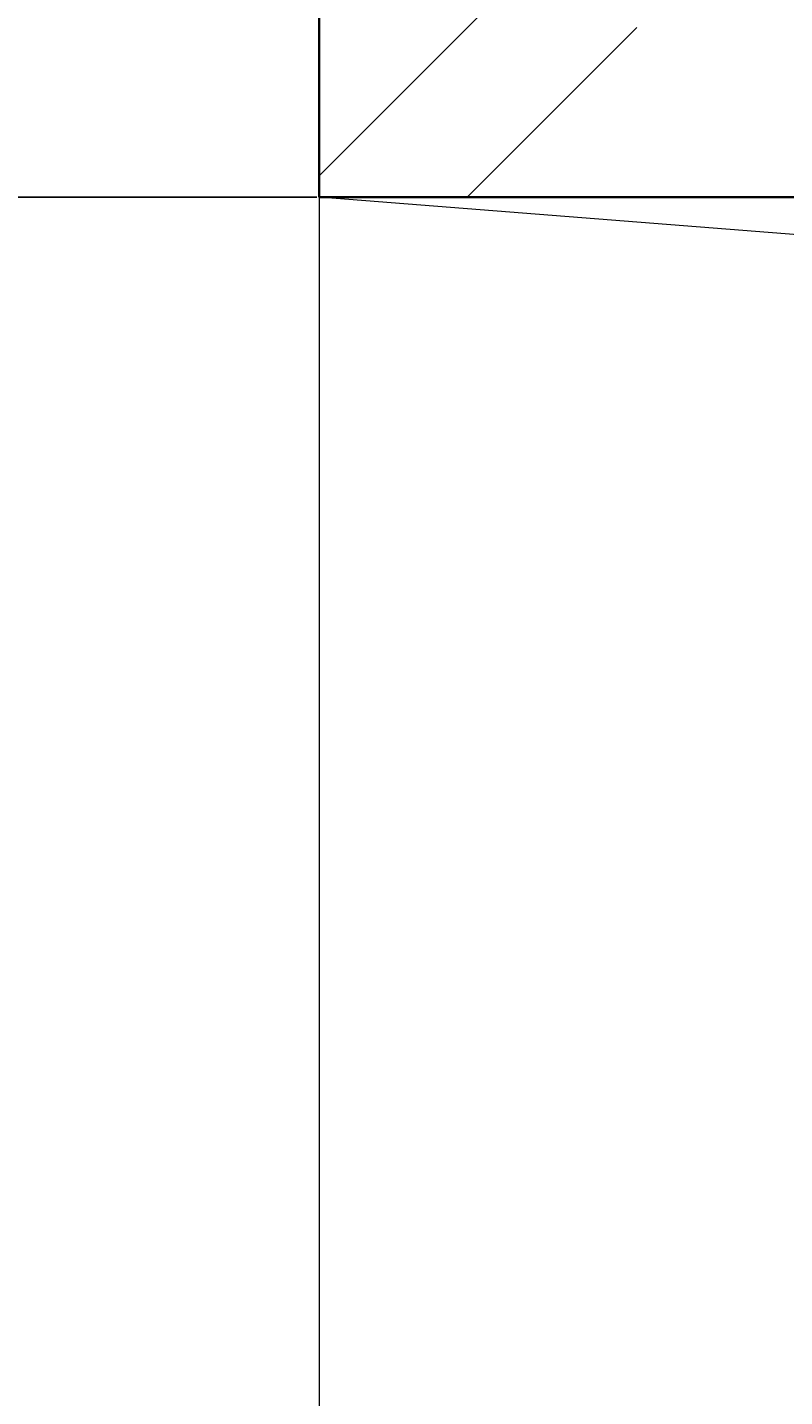
# Model space of a CAD drawing. Units: inches. Extents: x 1885 to 2748, y 783 to 2421.
# Tile 57 of 117: x 2009 to 2029, y 1850 to 1886. Entities that reach past the tile are written whole.
import ezdxf

# ---------------------------------------------------------------- set-up
doc = ezdxf.new("R2010")
doc.units = ezdxf.units.IN
for name, color, linetype, lineweight in [('A-ANNO-DIMS', 2, 'Continuous', 18), ('A-FLOR-OPEN', 8, 'Continuous', 13), ('A-WALL', 7, 'Continuous', 35)]:
    doc.layers.add(name, color=color, linetype=linetype, lineweight=lineweight)
doc.layers.add('A-WALL-PATT', color=85, linetype='Continuous', lineweight=13, true_color=0x58ba48)
doc.styles.get("Standard").update_dxf_attribs({"font": 'arial.ttf'})
doc.dimstyles.get("Standard").update_dxf_attribs({"dimtxt": 0.18, "dimasz": 0.18, "dimexe": 0.18, "dimexo": 0.0625, "dimgap": 0.09, "dimtad": 0, "dimtih": 1, "dimtoh": 1, "dimdec": 4, "dimzin": 0, "dimdsep": 46, "dimtxsty": 'Standard', "dimcen": 0.09, "dimadec": 0, "dimazin": 0, "dimtfac": 1, "dimtdec": 4, "dimtofl": 0, "dimtmove": 0, "dimatfit": 3, "dimfxl": 1, "dimtolj": 1, "dimtzin": 0, "dimarcsym": 0})

# ---------------------------------------------------------------- blocks, each defined once
blk = doc.blocks.new('*D48')
at = {"layer": 'A-ANNO-DIMS', "color": 0, "lineweight": -2, "transparency": 16777216}
for p, q in [((1980.711, 2348.006), (1902.844, 2348.006)), ((1903.024, 2347.826), (1903.024, 2114.937)), ((1903.024, 1881.686), (1903.024, 2114.574)), ((2016.711, 1881.506), (1902.844, 1881.506))]:
    blk.add_line(p, q, dxfattribs=at)
at = {"layer": 'A-ANNO-DIMS', "color": 0, "transparency": 16777216}
for points in [[(1902.994, 2347.826), (1903.054, 2347.826), (1903.024, 2348.006)], [(1902.994, 1881.686), (1903.054, 1881.686), (1903.024, 1881.506)]]:
    blk.add_solid(points, dxfattribs=at)
at = {"layer": 'Defpoints', "color": 0, "transparency": 16777216}
for p in [(1903.024, 2348.006), (1980.774, 2348.006), (2016.774, 1881.506)]:
    blk.add_point(p, dxfattribs=at)
at = {"layer": 'A-ANNO-DIMS', "color": 0, "transparency": 16777216, "insert": (1903.024, 2114.756), "char_height": 0.18, "attachment_point": 5}
blk.add_mtext('\\A1;466.5', dxfattribs=at)

msp = doc.modelspace()

# ---------------------------------------------------------------- hatches: boundary and pattern name
at = {"layer": 'A-WALL-PATT'}
h = msp.add_hatch(dxfattribs=at)
h.set_pattern_fill('ANSI32', color=256)
h.paths.add_polyline_path([(2007.772, 2318.006), (1980.774, 2318.006), (1980.774, 2281.215), (1985.274, 2281.215), (1985.274, 2313.506), (2007.772, 2313.506), (2007.772, 2315.756)])
h.paths.add_polyline_path([(2094.324, 2318.006), (2067.772, 2318.006), (2067.772, 2313.506), (2094.324, 2313.506), (2094.324, 2315.756)])
h.paths.add_polyline_path([(2131.367, 2315.756), (2131.367, 2318.006), (2131.189, 2318.006), (2112.609, 2318.006), (2112.609, 2313.506), (2117.274, 2313.506), (2117.274, 2255.201), (2121.774, 2255.201), (2121.774, 2313.506), (2131.367, 2313.506)])
h.paths.add_polyline_path([(2190.512, 2318.006), (2155.367, 2318.006), (2155.367, 2313.506), (2169.774, 2313.506), (2169.774, 2229.506), (2121.774, 2229.506), (2121.774, 2233.451), (2119.524, 2233.451), (2117.274, 2233.451), (2117.274, 2201.101), (2121.774, 2201.101), (2121.774, 2225.006), (2169.774, 2225.006), (2169.774, 2165.006), (2306.274, 2165.006), (2306.274, 2066.006), (2310.774, 2066.006), (2344.274, 2066.006), (2486.274, 2066.006), (2486.274, 1886.006), (2483.02, 1886.006), (2483.02, 1881.506), (2486.274, 1881.506), (2486.274, 1880.678), (2490.774, 1880.678), (2490.774, 2070.506), (2344.274, 2070.506), (2310.774, 2070.506), (2310.774, 2165.006), (2310.774, 2173.636), (2308.524, 2173.636), (2306.274, 2173.636), (2306.274, 2169.506), (2174.274, 2169.506), (2174.274, 2313.506), (2190.512, 2313.506), (2190.512, 2315.756)])
h.paths.add_polyline_path([(1985.274, 2221.215), (1980.774, 2221.215), (1980.774, 2165.006), (1992.774, 2165.006), (1992.774, 2141.927), (1997.274, 2141.927), (1997.274, 2165.006), (2117.274, 2165.006), (2117.274, 2163.126), (2121.774, 2163.126), (2121.774, 2172.734), (2119.524, 2172.734), (2117.274, 2172.734), (2117.274, 2169.506), (1985.274, 2169.506)])
h.paths.add_polyline_path([(1997.274, 2105.927), (1992.774, 2105.927), (1992.774, 2070.506), (2016.774, 2070.506), (2016.774, 2059.123), (2019.024, 2059.123), (2021.274, 2059.123), (2021.274, 2070.506), (2117.274, 2070.506), (2117.274, 2022.506), (2114.423, 2022.506), (2114.423, 2018.006), (2123.627, 2018.006), (2123.627, 2020.256), (2123.627, 2022.506), (2121.774, 2022.506), (2121.774, 2142.587), (2119.524, 2142.587), (2117.274, 2142.587), (2117.274, 2075.006), (1997.274, 2075.006)])
h.paths.add_polyline_path([(2092.029, 2020.256), (2092.029, 2022.506), (2021.274, 2022.506), (2021.274, 2035.123), (2016.774, 2035.123), (2016.774, 2018.006), (2016.774, 1978.784), (2021.274, 1978.784), (2021.274, 2018.006), (2092.029, 2018.006)])
h.paths.add_polyline_path([(2260.938, 2022.506), (2153.105, 2022.506), (2153.105, 2020.256), (2153.105, 2018.006), (2155.274, 2018.006), (2155.274, 1886.006), (2107.629, 1886.006), (2107.629, 1881.506), (2182.911, 1881.506), (2182.911, 1883.756), (2182.911, 1886.006), (2159.774, 1886.006), (2159.774, 2018.006), (2260.938, 2018.006), (2260.938, 2020.256)])
h.paths.add_polyline_path([(2047.629, 1883.756), (2047.629, 1886.006), (2021.274, 1886.006), (2021.274, 1918.784), (2019.024, 1918.784), (2016.774, 1918.784), (2016.774, 1881.506), (2047.629, 1881.506)])
h.paths.add_polyline_path([(2306.361, 1883.756), (2306.361, 1886.006), (2296.274, 1886.006), (2296.274, 1982.006), (2316.535, 1982.006), (2316.535, 1984.256), (2316.535, 1986.506), (2296.274, 1986.506), (2296.274, 2022.506), (2289.276, 2022.506), (2289.276, 2018.006), (2291.774, 2018.006), (2291.774, 1886.006), (2242.911, 1886.006), (2242.911, 1881.506), (2306.361, 1881.506)], flags=17)
h.paths.add_polyline_path([(1985.274, 1843.006), (2021.6, 1843.006), (2021.534, 1845.441), (2021.477, 1847.506), (1980.774, 1847.506), (1980.774, 1809.446), (1985.274, 1809.446)])
h.paths.add_polyline_path([(2131.482, 1845.256), (2131.482, 1847.506), (2081.534, 1847.506), (2081.534, 1843.006), (2117.274, 1843.006), (2117.274, 1784.147), (2119.524, 1784.147), (2121.774, 1784.147), (2121.774, 1843.006), (2131.482, 1843.006)])
h.paths.add_polyline_path([(2203.886, 1847.506), (2155.482, 1847.506), (2155.482, 1843.006), (2169.774, 1843.006), (2169.774, 1759.006), (2121.774, 1759.006), (2121.774, 1761.457), (2117.274, 1761.457), (2117.274, 1730.429), (2121.774, 1730.429), (2121.774, 1754.506), (2177.421, 1754.506), (2177.421, 1756.756), (2177.421, 1759.006), (2174.274, 1759.006), (2174.274, 1843.006), (2203.886, 1843.006)])
h.paths.add_polyline_path([(2335.554, 1845.256), (2335.554, 1847.506), (2239.886, 1847.506), (2239.886, 1843.006), (2306.274, 1843.006), (2306.274, 1759.006), (2199.486, 1759.006), (2199.486, 1754.506), (2310.774, 1754.506), (2310.774, 1843.006), (2335.554, 1843.006)])
h.paths.add_polyline_path([(2348.774, 2022.506), (2344.274, 2022.506), (2344.274, 1986.506), (2341.681, 1986.506), (2341.681, 1982.006), (2344.274, 1982.006), (2344.274, 1886.006), (2330.361, 1886.006), (2330.361, 1881.506), (2361.627, 1881.506), (2361.627, 1883.756), (2361.627, 1886.006), (2348.774, 1886.006)], flags=17)
h.paths.add_polyline_path([(2283.251, 2315.756), (2283.251, 2318.006), (2238.512, 2318.006), (2238.512, 2313.506), (2283.251, 2313.506)], flags=17)
h.paths.add_polyline_path([(2363.274, 2348.006), (2388.677, 2348.006), (2388.677, 2350.256), (2388.677, 2352.506), (2358.774, 2352.506), (2358.774, 2348.006), (2358.774, 2318.006), (2344.481, 2318.006), (2344.481, 2313.506), (2358.774, 2313.506), (2358.774, 2229.506), (2310.774, 2229.506), (2310.774, 2231.952), (2306.274, 2231.952), (2306.274, 2205.611), (2310.774, 2205.611), (2310.774, 2225.006), (2358.774, 2225.006), (2358.774, 2211.506), (2452.329, 2211.506), (2452.329, 2213.756), (2452.329, 2216.006), (2363.274, 2216.006), (2363.274, 2318.006)])
h.paths.add_polyline_path([(2310.774, 2313.506), (2320.481, 2313.506), (2320.481, 2315.756), (2320.481, 2318.006), (2302.728, 2318.006), (2302.728, 2313.506), (2306.274, 2313.506), (2306.274, 2251.076), (2310.774, 2251.076)], flags=17)
h.paths.add_polyline_path([(2490.774, 2352.506), (2486.274, 2352.506), (2448.677, 2352.506), (2448.677, 2348.006), (2486.274, 2348.006), (2486.274, 2318.006), (2486.274, 2216.006), (2481.78, 2216.006), (2481.78, 2211.506), (2486.274, 2211.506), (2486.274, 2165.006), (2493.289, 2165.006), (2493.289, 2167.256), (2493.289, 2169.506), (2490.774, 2169.506), (2490.774, 2313.506), (2494.429, 2313.506), (2494.429, 2318.006), (2490.774, 2318.006)])
h.paths.add_polyline_path([(2534.653, 2318.006), (2515.691, 2318.006), (2515.691, 2313.506), (2534.653, 2313.506), (2534.653, 2315.756)])
h.paths.add_polyline_path([(2618.274, 2318.006), (2594.653, 2318.006), (2594.653, 2313.506), (2613.774, 2313.506), (2613.774, 2281.706), (2618.274, 2281.706)])
h.paths.add_polyline_path([(2618.274, 2221.706), (2613.774, 2221.706), (2613.774, 2169.506), (2554.019, 2169.506), (2554.019, 2165.006), (2613.774, 2165.006), (2613.774, 2152.878), (2618.274, 2152.878)])
h.paths.add_polyline_path([(2618.274, 2128.878), (2616.024, 2128.878), (2613.774, 2128.878), (2613.774, 2117.006), (2529.774, 2117.006), (2529.774, 2165.006), (2532.848, 2165.006), (2532.848, 2169.506), (2522.867, 2169.506), (2522.867, 2165.006), (2525.274, 2165.006), (2525.274, 2117.006), (2525.274, 2112.506), (2525.274, 2108.576), (2529.774, 2108.576), (2529.774, 2112.506), (2613.774, 2112.506), (2613.774, 2080.19), (2618.274, 2080.19)])
h.paths.add_polyline_path([(2618.274, 2044.19), (2616.024, 2044.19), (2613.774, 2044.19), (2613.774, 2015.506), (2529.774, 2015.506), (2529.774, 2088.582), (2527.524, 2088.582), (2525.274, 2088.582), (2525.274, 2011.006), (2613.774, 2011.006), (2613.774, 1956.755), (2618.274, 1956.755)])
h.paths.add_polyline_path([(2618.274, 1881.506), (2618.274, 1896.755), (2613.774, 1896.755), (2613.774, 1881.506), (2613.774, 1847.506), (2592.715, 1847.506), (2592.715, 1843.006), (2613.774, 1843.006), (2613.774, 1765.006), (2613.774, 1760.506), (2609.621, 1760.506), (2609.621, 1756.006), (2613.774, 1756.006), (2613.774, 1660.006), (2608.544, 1660.006), (2608.544, 1655.506), (2613.774, 1655.506), (2613.774, 1508.158), (2618.274, 1508.158)])
h.paths.add_polyline_path([(2565.774, 1843.006), (2568.997, 1843.006), (2568.997, 1847.506), (2490.774, 1847.506), (2490.774, 1849.7), (2488.524, 1849.7), (2486.274, 1849.7), (2486.274, 1847.506), (2477.274, 1847.506), (2477.274, 1838.506), (2477.274, 1821.493), (2486.274, 1821.493), (2486.274, 1838.506), (2561.274, 1838.506), (2561.274, 1765.006), (2486.274, 1765.006), (2486.274, 1786.157), (2477.274, 1786.157), (2477.274, 1765.006), (2477.274, 1756.006), (2486.274, 1756.006), (2565.774, 1756.006), (2585.621, 1756.006), (2585.621, 1758.256), (2585.621, 1760.506), (2565.774, 1760.506), (2565.774, 1765.006)])
h.paths.add_polyline_path([(2486.274, 1651.006), (2561.274, 1651.006), (2561.274, 1567.006), (2486.274, 1567.006), (2486.274, 1591.321), (2477.274, 1591.321), (2477.274, 1567.006), (2477.274, 1558.006), (2477.274, 1555.439), (2481.774, 1555.439), (2481.774, 1558.006), (2568.653, 1558.006), (2568.653, 1560.256), (2568.653, 1562.506), (2565.774, 1562.506), (2565.774, 1655.506), (2584.544, 1655.506), (2584.544, 1657.756), (2584.544, 1660.006), (2565.774, 1660.006), (2486.274, 1660.006), (2477.274, 1660.006), (2477.274, 1651.006), (2477.274, 1632.989), (2486.274, 1632.989)])
h.paths.add_polyline_path([(2449.967, 1883.756), (2449.967, 1886.006), (2421.627, 1886.006), (2421.627, 1881.506), (2449.967, 1881.506)], flags=17)
h.paths.add_polyline_path([(2447.274, 1847.506), (2395.554, 1847.506), (2395.554, 1843.006), (2442.774, 1843.006), (2442.774, 1809.27), (2447.274, 1809.27)])
h.paths.add_polyline_path([(1985.274, 1749.446), (1980.774, 1749.446), (1980.774, 1694.504), (1985.274, 1694.504), (1985.274, 1694.506), (1986.897, 1694.506), (1986.897, 1697.78), (1986.897, 1699.006), (1985.274, 1699.006)])
h.paths.add_polyline_path([(2152.774, 1699.006), (2121.774, 1699.006), (2121.774, 1703.668), (2119.524, 1703.668), (2117.274, 1703.668), (2117.274, 1699.006), (2009.219, 1699.006), (2009.219, 1694.506), (2148.274, 1694.506), (2148.274, 1692.631), (2152.774, 1692.631)])
h.paths.add_polyline_path([(2016.274, 1694.506), (2011.774, 1694.506), (2011.774, 1558.006), (2040.806, 1558.006), (2040.806, 1560.256), (2040.806, 1562.506), (2016.274, 1562.506)])
h.paths.add_polyline_path([(2152.774, 1663.017), (2150.524, 1663.017), (2148.274, 1663.017), (2148.274, 1562.506), (2100.806, 1562.506), (2100.806, 1558.006), (2165.119, 1558.006), (2165.119, 1560.256), (2165.119, 1562.506), (2152.774, 1562.506), (2152.774, 1610.506), (2224.774, 1610.506), (2224.774, 1607.99), (2229.274, 1607.99), (2229.274, 1615.006), (2152.774, 1615.006)])
h.paths.add_polyline_path([(2238.613, 1560.256), (2238.613, 1562.506), (2229.274, 1562.506), (2229.274, 1588.756), (2227.024, 1588.763), (2224.774, 1588.771), (2224.774, 1562.506), (2189.119, 1562.506), (2189.119, 1558.006), (2238.613, 1558.006)])
h.paths.add_polyline_path([(2336.024, 1560.256), (2336.024, 1562.506), (2310.774, 1562.506), (2310.774, 1656.347), (2308.524, 1656.347), (2306.274, 1656.347), (2306.274, 1562.506), (2286.613, 1562.506), (2286.613, 1558.006), (2336.024, 1558.006)])
h.paths.add_polyline_path([(2447.274, 1690.968), (2445.024, 1690.968), (2442.774, 1690.968), (2442.774, 1687.006), (2306.274, 1687.006), (2306.274, 1680.75), (2310.774, 1680.75), (2310.774, 1682.506), (2442.774, 1682.506), (2442.774, 1562.506), (2396.024, 1562.506), (2396.024, 1558.006), (2447.274, 1558.006)])
h.paths.add_polyline_path([(2447.274, 1749.27), (2445.024, 1749.27), (2442.774, 1749.27), (2442.774, 1717.232), (2447.274, 1717.232)])
h.paths.add_polyline_path([(2044.674, 1521.756), (2044.674, 1524.006), (2007.274, 1524.006), (2007.274, 1503.49), (2009.524, 1503.49), (2011.774, 1503.49), (2011.774, 1519.506), (2044.674, 1519.506)])
h.paths.add_polyline_path([(2177.969, 1521.756), (2177.969, 1524.006), (2104.674, 1524.006), (2104.674, 1519.506), (2145.774, 1519.506), (2145.774, 1387.506), (2143.37, 1387.506), (2143.37, 1383.006), (2251.585, 1383.006), (2251.585, 1385.256), (2251.585, 1387.506), (2150.274, 1387.506), (2150.274, 1519.506), (2177.969, 1519.506)])
h.paths.add_polyline_path([(2298.704, 1524.006), (2237.969, 1524.006), (2237.969, 1519.506), (2282.274, 1519.506), (2282.274, 1387.506), (2279.683, 1387.506), (2279.683, 1383.006), (2286.774, 1383.006), (2286.774, 1419.006), (2312.451, 1419.006), (2312.451, 1421.256), (2312.451, 1423.506), (2286.774, 1423.506), (2286.774, 1519.506), (2298.704, 1519.506), (2298.704, 1521.722)], flags=17)
h.paths.add_polyline_path([(2361.897, 1521.756), (2361.897, 1524.006), (2322.704, 1524.006), (2322.704, 1519.506), (2334.774, 1519.506), (2334.774, 1423.506), (2331.93, 1423.506), (2331.93, 1419.006), (2334.774, 1419.006), (2334.774, 1387.506), (2334.774, 1383.228), (2339.274, 1383.228), (2339.274, 1387.506), (2339.274, 1519.506), (2361.897, 1519.506)], flags=17)
h.paths.add_polyline_path([(2447.274, 1521.756), (2447.274, 1524.006), (2421.897, 1524.006), (2421.897, 1519.506), (2447.274, 1519.506)], flags=17)
h.paths.add_polyline_path([(2481.774, 1529.6), (2479.524, 1529.6), (2477.274, 1529.6), (2477.274, 1524.006), (2474.489, 1524.006), (2474.489, 1519.506), (2477.274, 1519.506), (2477.274, 1334.506), (2296.774, 1334.506), (2296.774, 1240.506), (2160.274, 1240.506), (2160.274, 1180.506), (2112.274, 1180.506), (2112.274, 1207.692), (2110.024, 1207.692), (2107.774, 1207.692), (2107.774, 1171.609), (2112.274, 1171.609), (2112.274, 1176.006), (2160.274, 1176.006), (2160.274, 1092.006), (2144.221, 1092.006), (2144.221, 1087.506), (2189.497, 1087.506), (2189.497, 1089.756), (2189.497, 1092.006), (2164.774, 1092.006), (2164.774, 1236.006), (2296.774, 1236.006), (2296.774, 1231.912), (2301.274, 1231.912), (2301.274, 1330.006), (2481.774, 1330.006), (2481.774, 1387.506)])
h.paths.add_polyline_path([(2618.274, 1448.158), (2613.774, 1448.158), (2613.774, 1382.506), (2529.774, 1382.506), (2525.274, 1382.506), (2525.274, 1307.062), (2529.774, 1307.062), (2529.774, 1378.006), (2613.774, 1378.006), (2613.774, 1354.988), (2618.274, 1354.988)])
h.paths.add_polyline_path([(2618.274, 1318.988), (2613.774, 1318.988), (2613.774, 1281.006), (2529.774, 1281.006), (2529.774, 1283.786), (2527.524, 1283.786), (2525.274, 1283.786), (2525.274, 1228.506), (2516.794, 1228.506), (2516.794, 1224.006), (2533.484, 1224.006), (2533.484, 1226.256), (2533.484, 1228.506), (2529.774, 1228.506), (2529.774, 1276.506), (2613.774, 1276.506), (2613.774, 1266.02), (2618.274, 1266.02)])
h.paths.add_polyline_path([(2618.274, 1134.964), (2613.774, 1134.964), (2613.774, 1092.006), (2594.545, 1092.006), (2594.545, 1087.506), (2618.274, 1087.506)])
h.paths.add_polyline_path([(2534.545, 1092.006), (2509.765, 1092.006), (2509.765, 1087.506), (2534.545, 1087.506), (2534.545, 1089.756)])
h.paths.add_polyline_path([(2481.274, 1224.006), (2484.117, 1224.006), (2484.117, 1226.256), (2484.117, 1228.506), (2476.774, 1228.506), (2476.774, 1198.506), (2471.61, 1198.506), (2471.61, 1194.006), (2476.774, 1194.006), (2476.774, 1062.006), (2436.894, 1062.006), (2436.894, 1057.506), (2476.774, 1057.506), (2481.274, 1057.506), (2481.274, 1062.006), (2481.274, 1087.506), (2485.354, 1087.506), (2485.354, 1089.756), (2485.354, 1092.006), (2481.274, 1092.006), (2481.274, 1117.506)])
h.paths.add_polyline_path([(2439.898, 1198.506), (2349.274, 1198.506), (2349.274, 1194.006), (2349.274, 1180.506), (2301.274, 1180.506), (2301.274, 1201.896), (2299.024, 1201.896), (2296.774, 1201.896), (2296.774, 1172.335), (2299.024, 1172.335), (2301.274, 1172.335), (2301.274, 1176.006), (2349.274, 1176.006), (2349.274, 1092.006), (2334.452, 1092.006), (2334.452, 1087.506), (2349.274, 1087.506), (2349.274, 1057.506), (2353.774, 1057.506), (2376.894, 1057.506), (2376.894, 1059.756), (2376.894, 1062.006), (2353.774, 1062.006), (2353.774, 1087.506), (2353.774, 1180.506), (2353.774, 1194.006), (2439.898, 1194.006), (2439.898, 1196.256)])
h.paths.add_polyline_path([(2270.596, 1089.756), (2270.596, 1092.006), (2249.497, 1092.006), (2249.497, 1087.506), (2270.596, 1087.506)], flags=17)
h.paths.add_polyline_path([(2310.452, 1092.006), (2301.274, 1092.006), (2301.274, 1153.292), (2296.774, 1153.292), (2296.774, 1092.006), (2293.786, 1092.006), (2293.786, 1087.506), (2310.452, 1087.506), (2310.452, 1089.756)], flags=17)
h.paths.add_polyline_path([(2112.274, 1150.328), (2110.024, 1150.328), (2107.774, 1150.328), (2107.774, 1092.006), (2104.465, 1092.006), (2104.465, 1087.506), (2120.221, 1087.506), (2120.221, 1089.756), (2120.221, 1092.006), (2112.274, 1092.006)])
h.paths.add_polyline_path([(2082.172, 1092.006), (2058.144, 1092.006), (2058.144, 1087.506), (2082.172, 1087.506), (2082.172, 1089.756)])
h.paths.add_polyline_path([(1975.774, 1145.638), (1971.274, 1145.638), (1971.274, 1087.506), (1980.774, 1087.506), (1998.144, 1087.506), (1998.144, 1089.756), (1998.144, 1092.006), (1985.274, 1092.006), (1975.774, 1092.006)])
h.paths.add_polyline_path([(2112.274, 1244.385), (2110.024, 1244.385), (2107.774, 1244.385), (2107.774, 1240.506), (1992.274, 1240.506), (1992.274, 1271.008), (1987.774, 1271.008), (1987.774, 1240.506), (1980.774, 1240.506), (1975.774, 1240.506), (1971.274, 1240.506), (1971.274, 1205.638), (1975.774, 1205.638), (1975.774, 1236.006), (2107.774, 1236.006), (2107.774, 1233.444), (2112.274, 1233.444), (2112.274, 1236.006)])
h.paths.add_polyline_path([(2112.274, 1383.006), (2114.783, 1383.006), (2114.783, 1385.256), (2114.783, 1387.506), (2102.476, 1387.506), (2102.476, 1383.006), (2107.774, 1383.006), (2107.774, 1335.006), (2011.774, 1335.006), (2011.774, 1349.939), (2007.274, 1349.939), (2007.274, 1335.006), (1987.774, 1335.006), (1987.774, 1330.506), (1987.774, 1307.008), (1992.274, 1307.008), (1992.274, 1330.506), (2007.274, 1330.506), (2107.774, 1330.506), (2107.774, 1264.711), (2112.274, 1264.711)])
h.paths.add_polyline_path([(2077.857, 1387.506), (2011.774, 1387.506), (2011.774, 1390.036), (2009.524, 1390.036), (2007.274, 1390.036), (2007.274, 1373.939), (2011.774, 1373.939), (2011.774, 1383.006), (2077.857, 1383.006)])
h.paths.add_polyline_path([(2011.774, 1443.49), (2007.274, 1443.49), (2007.274, 1410.248), (2011.774, 1410.248)])

# ---------------------------------------------------------------- linework, layer by layer
at = {"layer": 'A-FLOR-OPEN'}
for p, q in [((2016.774, 1881.506), (2016.774, 1847.506)), ((2447.274, 1847.506), (2016.774, 1881.506))]:
    msp.add_line(p, q, dxfattribs=at)
at = {"layer": 'A-WALL'}
for p, q in [((2016.774, 1918.784), (2016.774, 1881.506)), ((2016.774, 1881.506), (2047.629, 1881.506)), ((2016.774, 1881.506), (2021.274, 1881.506)), ((2016.774, 1881.506), (2047.629, 1881.506))]:
    msp.add_line(p, q, dxfattribs=at)

# ---------------------------------------------------------------- dimensions: what is measured, and where the dimension line sits
at = {"layer": 'A-ANNO-DIMS'}
dim = msp.add_linear_dim(base=(1903.024, 2348.006), p1=(2016.774, 1881.506), p2=(1980.774, 2348.006), angle=90, dimstyle='Standard', override={"dimdec": 1, "dimlfac": 1, "dimrnd": 0, "dimzin": 0, "dimdsep": 46, "dimlunit": 2}, dxfattribs=at)
dim.commit()
dim.dimension.update_dxf_attribs({"geometry": '*D48', "text_midpoint": (1903.024, 2114.756)})

doc.saveas('drawing.dxf')
